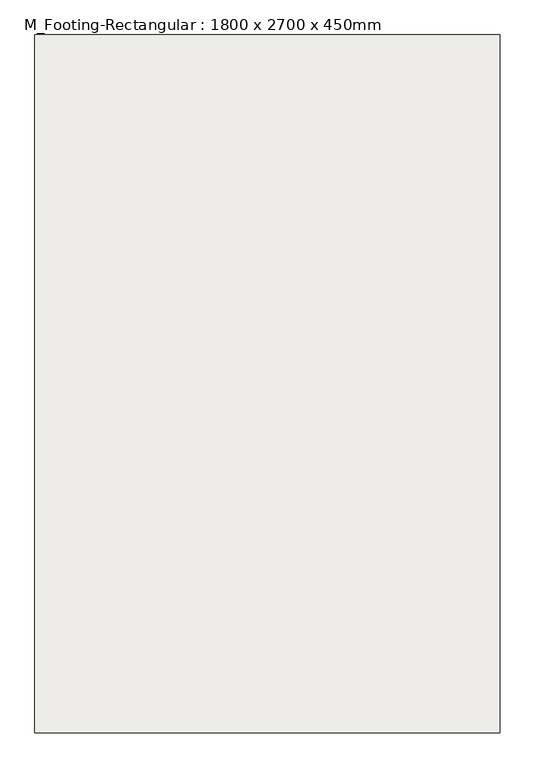
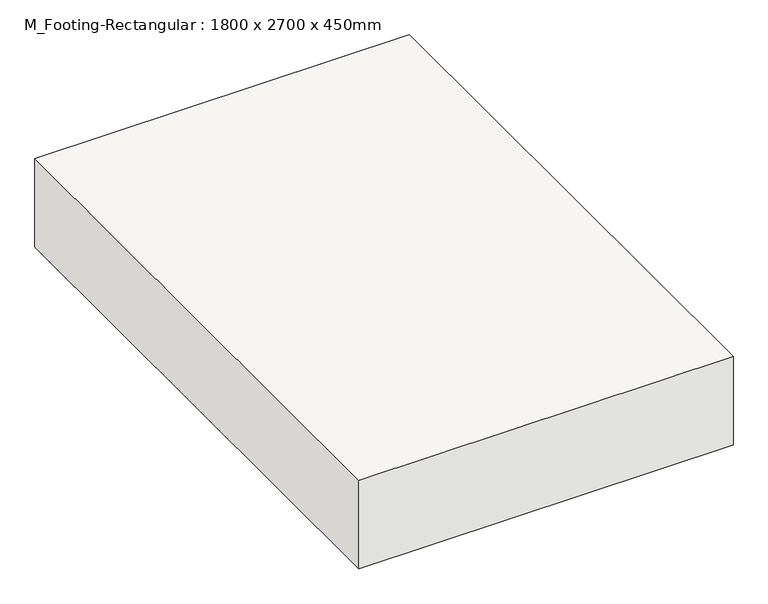
"""IFC4 building model written with IfcOpenShell, lengths in millimetres: slab geometry, M_Footing-Rectangular : 1800 x 2700 x 450mm."""

from ifc_helpers import new_model, si_unit, frame, origin, place, context, project, spatial, polyline, outline, extrude, source, transform, mapped, element, save


def m_footing_rectangular_1800_x_2700_x_450mm_20c57781(model_context):
    return source(origin(), model_context, "Body", "SweptSolid", [
        extrude(outline(polyline([(900.0, 1350.0), (900.0, -1350.0), (-900.0, -1350.0), (-900.0, 1350.0), (900.0, 1350.0)])), frame((0.0, 0.0, -450.0), z_axis=(0.0, 0.0, 1.0), x_axis=(1.0, 0.0, 0.0)), (0.0, 0.0, 1.0), 450.0),
    ])


if __name__ == "__main__":
    model = new_model("IFC4")
    model_context = context("Model", 3, world=origin())
    ifc_project = project(units=[si_unit("LENGTHUNIT", "METRE", prefix="MILLI")], contexts=[model_context])
    site = spatial("IfcSite", under=ifc_project)
    building = spatial("IfcBuilding", under=site)
    placement = place(None, origin())
    m_footing_rectangular_1800_x_2700_x_450mm_shape = m_footing_rectangular_1800_x_2700_x_450mm_20c57781(model_context)
    element("IfcSlab", 1, ObjectType="M_Footing-Rectangular : 1800 x 2700 x 450mm", at=placement, inside=building, context=model_context, shape_type="MappedRepresentation", body=[
        mapped(m_footing_rectangular_1800_x_2700_x_450mm_shape, transform((0.0, 0.0, 0.0), x_axis=(1.0, 0.0, 0.0), y_axis=(0.0, 1.0, 0.0), z_axis=(0.0, 0.0, 1.0))),
    ])
    save(model, "model.ifc")

# Revit data of these elements
# Type "M_Footing-Rectangular : 1800 x 2700 x 450mm"
#   Width = 5' - 10.86614"
#   Length = 8' - 10.29921"
#   Foundation Thickness = 1' - 5.71654"
#   Structural Material [instance default] = Concrete, Cast-in-Place gray
#   Assembly Code = ""
# Element 1 (IfcSlab, "M_Footing-Rectangular : 1800 x 2700 x 450mm")
#   Materials on its faces: "Concrete, Cast-in-Place gray"
# Materials
#   "Concrete, Cast-in-Place gray": class "Concrete", colour RGB 192 192 192, transparency 0, Description = "Cast-in-place concrete", Cost = 0
